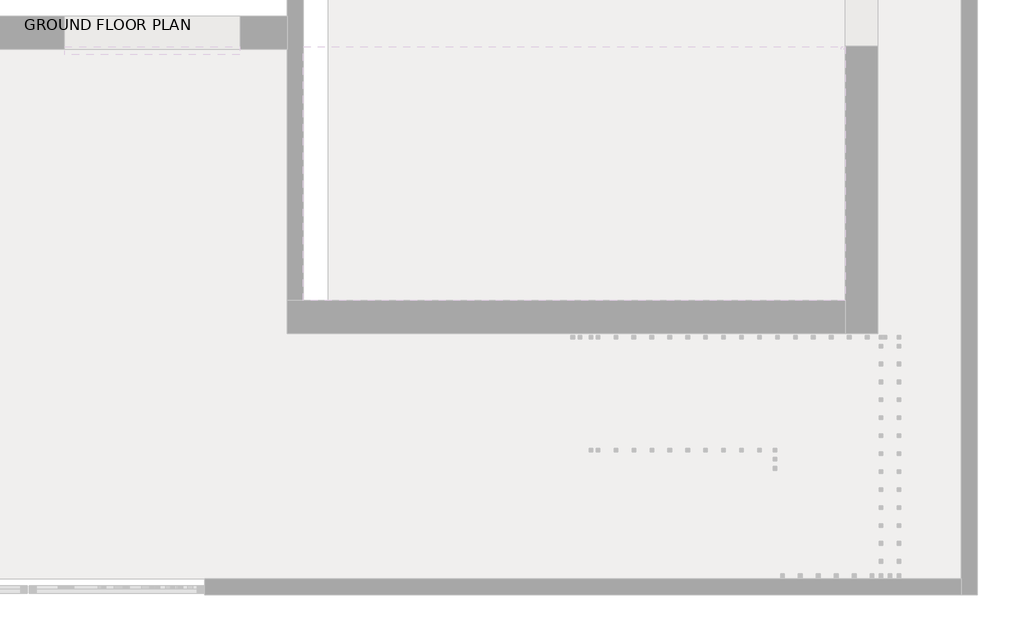
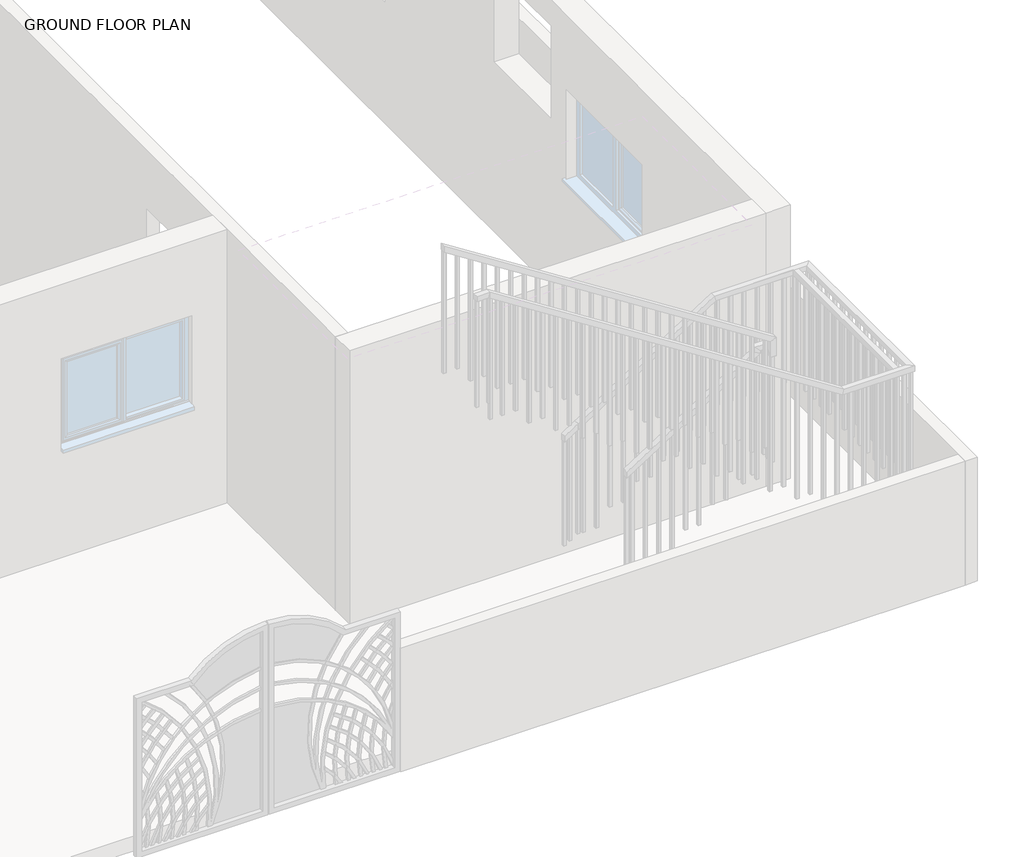
# One storey, part 13 of 23: 2 railings.
"""IFC4 building model written with IfcOpenShell, lengths in millimetres."""

from ifc_helpers import new_model, si_unit, frame, origin, place, context, project, spatial, polyline, outline, extrude, faceted_brep, element, save

model = new_model("IFC4")

# Units and contexts
model_context = context("Model", 3, world=origin())
ifc_project = project(units=[si_unit("LENGTHUNIT", "METRE", prefix="MILLI")], contexts=[model_context])

# Site, building, storey
site = spatial("IfcSite", under=ifc_project)
building = spatial("IfcBuilding", under=site)
storey = spatial("IfcBuildingStorey", under=building, Name="GROUND FLOOR PLAN", Elevation=487.68)

# Railings
placement = place(None, origin())
element("IfcRailing", 1, ObjectType="1100mm", at=placement, inside=storey, context=model_context, shape_type="SolidModel", body=[
    faceted_brep([(-8680.149573, -10220.0521308, 1912.8), (-8680.149573, -10220.0521308, 1853.4423995), (-8680.149573, -10270.0521308, 1853.4423995), (-8680.149573, -10270.0521308, 1912.8), (-7409.7306254, -10220.0521308, 2725.6), (-7395.1045513, -10220.0521308, 2675.6), (-7395.1045513, -10270.0521308, 2675.6), (-7409.7306254, -10270.0521308, 2725.6), (-6495.8132565, -10220.0521308, 2725.6), (-6495.8132565, -10220.0521308, 2675.6), (-6545.8132565, -10270.0521308, 2675.6), (-6545.8132565, -10270.0521308, 2725.6), (-6495.8132565, -11933.6860066, 2725.6), (-6495.8132565, -11933.6860066, 2675.6), (-6545.8132565, -11883.6860066, 2675.6), (-6545.8132565, -11883.6860066, 2725.6), (-7155.718398, -11933.6860066, 2725.6), (-7170.3479429, -11933.6860066, 2675.6), (-7170.3479429, -11883.6860066, 2675.6), (-7155.718398, -11883.6860066, 2725.6), (-10457.8773536, -11933.6860066, 4838.88), (-10457.8773536, -11883.6860066, 4838.88), (-10457.8773536, -11883.6860066, 4779.517542), (-10457.8773536, -11933.6860066, 4779.517542)], [[[0, 1, 2, 3]], [[1, 0, 4, 5]], [[2, 1, 5, 6]], [[3, 2, 6, 7]], [[0, 3, 7, 4]], [[5, 4, 8, 9]], [[6, 5, 9, 10]], [[7, 6, 10, 11]], [[4, 7, 11, 8]], [[9, 8, 12, 13]], [[10, 9, 13, 14]], [[11, 10, 14, 15]], [[8, 11, 15, 12]], [[13, 12, 16, 17]], [[14, 13, 17, 18]], [[15, 14, 18, 19]], [[12, 15, 19, 16]], [[20, 21, 22, 23]], [[17, 16, 20, 23]], [[18, 17, 23, 22]], [[19, 18, 22, 21]], [[16, 19, 21, 20]]]),
    extrude(outline(polyline([(4691.8007425, -10320.8132565), (4707.7999723, -10345.8132565), (3576.32, -10345.8132565), (3576.32, -10320.8132565), (4691.8007425, -10320.8132565)])), frame((0.0, -11921.1860066, 0.0), z_axis=(0.0, 1.0, 0.0), x_axis=(0.0, 0.0, 1.0)), (0.0, 0.0, 1.0), 25.0),
    extrude(outline(polyline([(4611.8045935, -10195.8132565), (4627.8038233, -10220.8132565), (3576.32, -10220.8132565), (3576.32, -10195.8132565), (4611.8045935, -10195.8132565)])), frame((0.0, -11921.1860066, 0.0), z_axis=(0.0, 1.0, 0.0), x_axis=(0.0, 0.0, 1.0)), (0.0, 0.0, 1.0), 25.0),
    extrude(outline(polyline([(4531.8084444, -10070.8132565), (4547.8076742, -10095.8132565), (3413.76, -10095.8132565), (3413.76, -10070.8132565), (4531.8084444, -10070.8132565)])), frame((0.0, -11921.1860066, 0.0), z_axis=(0.0, 1.0, 0.0), x_axis=(0.0, 0.0, 1.0)), (0.0, 0.0, 1.0), 25.0),
    extrude(outline(polyline([(4451.8122954, -9945.8132565), (4467.8115252, -9970.8132565), (3413.76, -9970.8132565), (3413.76, -9945.8132565), (4451.8122954, -9945.8132565)])), frame((0.0, -11921.1860066, 0.0), z_axis=(0.0, 1.0, 0.0), x_axis=(0.0, 0.0, 1.0)), (0.0, 0.0, 1.0), 25.0),
    extrude(outline(polyline([(4371.8161463, -9820.8132565), (4387.8153761, -9845.8132565), (3251.2, -9845.8132565), (3251.2, -9820.8132565), (4371.8161463, -9820.8132565)])), frame((0.0, -11921.1860066, 0.0), z_axis=(0.0, 1.0, 0.0), x_axis=(0.0, 0.0, 1.0)), (0.0, 0.0, 1.0), 25.0),
    extrude(outline(polyline([(4291.8423995, -9695.8132565), (4307.8371231, -9720.8132565), (3251.2, -9720.8132565), (3251.2, -9695.8132565), (4291.8423995, -9695.8132565)])), frame((0.0, -11921.1860066, 0.0), z_axis=(0.0, 1.0, 0.0), x_axis=(0.0, 0.0, 1.0)), (0.0, 0.0, 1.0), 25.0),
    extrude(outline(polyline([(4211.8238482, -9570.8132565), (4227.823078, -9595.8132565), (3088.64, -9595.8132565), (3088.64, -9570.8132565), (4211.8238482, -9570.8132565)])), frame((0.0, -11921.1860066, 0.0), z_axis=(0.0, 1.0, 0.0), x_axis=(0.0, 0.0, 1.0)), (0.0, 0.0, 1.0), 25.0),
    extrude(outline(polyline([(4131.8276992, -9445.8132565), (4147.826929, -9470.8132565), (3088.64, -9470.8132565), (3088.64, -9445.8132565), (4131.8276992, -9445.8132565)])), frame((0.0, -11921.1860066, 0.0), z_axis=(0.0, 1.0, 0.0), x_axis=(0.0, 0.0, 1.0)), (0.0, 0.0, 1.0), 25.0),
    extrude(outline(polyline([(4051.8315501, -9320.8132565), (4067.8307799, -9345.8132565), (2926.08, -9345.8132565), (2926.08, -9320.8132565), (4051.8315501, -9320.8132565)])), frame((0.0, -11921.1860066, 0.0), z_axis=(0.0, 1.0, 0.0), x_axis=(0.0, 0.0, 1.0)), (0.0, 0.0, 1.0), 25.0),
    extrude(outline(polyline([(3971.835401, -9195.8132565), (3987.8346309, -9220.8132565), (2926.08, -9220.8132565), (2926.08, -9195.8132565), (3971.835401, -9195.8132565)])), frame((0.0, -11921.1860066, 0.0), z_axis=(0.0, 1.0, 0.0), x_axis=(0.0, 0.0, 1.0)), (0.0, 0.0, 1.0), 25.0),
    extrude(outline(polyline([(3891.839252, -9070.8132565), (3907.8384818, -9095.8132565), (2763.52, -9095.8132565), (2763.52, -9070.8132565), (3891.839252, -9070.8132565)])), frame((0.0, -11921.1860066, 0.0), z_axis=(0.0, 1.0, 0.0), x_axis=(0.0, 0.0, 1.0)), (0.0, 0.0, 1.0), 25.0),
    extrude(outline(polyline([(3811.8431029, -8945.8132565), (3827.8423328, -8970.8132565), (2763.52, -8970.8132565), (2763.52, -8945.8132565), (3811.8431029, -8945.8132565)])), frame((0.0, -11921.1860066, 0.0), z_axis=(0.0, 1.0, 0.0), x_axis=(0.0, 0.0, 1.0)), (0.0, 0.0, 1.0), 25.0),
    extrude(outline(polyline([(3731.8469539, -8820.8132565), (3747.8461837, -8845.8132565), (2600.96, -8845.8132565), (2600.96, -8820.8132565), (3731.8469539, -8820.8132565)])), frame((0.0, -11921.1860066, 0.0), z_axis=(0.0, 1.0, 0.0), x_axis=(0.0, 0.0, 1.0)), (0.0, 0.0, 1.0), 25.0),
    extrude(outline(polyline([(3651.8508048, -8695.8132565), (3667.8500347, -8720.8132565), (2600.96, -8720.8132565), (2600.96, -8695.8132565), (3651.8508048, -8695.8132565)])), frame((0.0, -11921.1860066, 0.0), z_axis=(0.0, 1.0, 0.0), x_axis=(0.0, 0.0, 1.0)), (0.0, 0.0, 1.0), 25.0),
    extrude(outline(polyline([(3571.8546558, -8570.8132565), (3587.8538856, -8595.8132565), (2438.4, -8595.8132565), (2438.4, -8570.8132565), (3571.8546558, -8570.8132565)])), frame((0.0, -11921.1860066, 0.0), z_axis=(0.0, 1.0, 0.0), x_axis=(0.0, 0.0, 1.0)), (0.0, 0.0, 1.0), 25.0),
    extrude(outline(polyline([(3491.8585067, -8445.8132565), (3507.8577365, -8470.8132565), (2438.4, -8470.8132565), (2438.4, -8445.8132565), (3491.8585067, -8445.8132565)])), frame((0.0, -11921.1860066, 0.0), z_axis=(0.0, 1.0, 0.0), x_axis=(0.0, 0.0, 1.0)), (0.0, 0.0, 1.0), 25.0),
    extrude(outline(polyline([(3411.8623577, -8320.8132565), (3427.8615875, -8345.8132565), (2275.84, -8345.8132565), (2275.84, -8320.8132565), (3411.8623577, -8320.8132565)])), frame((0.0, -11921.1860066, 0.0), z_axis=(0.0, 1.0, 0.0), x_axis=(0.0, 0.0, 1.0)), (0.0, 0.0, 1.0), 25.0),
    extrude(outline(polyline([(3331.8662086, -8195.8132565), (3347.8654384, -8220.8132565), (2275.84, -8220.8132565), (2275.84, -8195.8132565), (3331.8662086, -8195.8132565)])), frame((0.0, -11921.1860066, 0.0), z_axis=(0.0, 1.0, 0.0), x_axis=(0.0, 0.0, 1.0)), (0.0, 0.0, 1.0), 25.0),
    extrude(outline(polyline([(3251.8700596, -8070.8132565), (3267.8692894, -8095.8132565), (2113.28, -8095.8132565), (2113.28, -8070.8132565), (3251.8700596, -8070.8132565)])), frame((0.0, -11921.1860066, 0.0), z_axis=(0.0, 1.0, 0.0), x_axis=(0.0, 0.0, 1.0)), (0.0, 0.0, 1.0), 25.0),
    extrude(outline(polyline([(3171.8739105, -7945.8132565), (3187.8731403, -7970.8132565), (2113.28, -7970.8132565), (2113.28, -7945.8132565), (3171.8739105, -7945.8132565)])), frame((0.0, -11921.1860066, 0.0), z_axis=(0.0, 1.0, 0.0), x_axis=(0.0, 0.0, 1.0)), (0.0, 0.0, 1.0), 25.0),
    extrude(outline(polyline([(3091.8777615, -7820.8132565), (3107.8769913, -7845.8132565), (1950.72, -7845.8132565), (1950.72, -7820.8132565), (3091.8777615, -7820.8132565)])), frame((0.0, -11921.1860066, 0.0), z_axis=(0.0, 1.0, 0.0), x_axis=(0.0, 0.0, 1.0)), (0.0, 0.0, 1.0), 25.0),
    extrude(outline(polyline([(3011.8816124, -7695.8132565), (3027.8808422, -7720.8132565), (1950.72, -7720.8132565), (1950.72, -7695.8132565), (3011.8816124, -7695.8132565)])), frame((0.0, -11921.1860066, 0.0), z_axis=(0.0, 1.0, 0.0), x_axis=(0.0, 0.0, 1.0)), (0.0, 0.0, 1.0), 25.0),
    extrude(outline(polyline([(2931.8854634, -7570.8132565), (2947.8846932, -7595.8132565), (1788.16, -7595.8132565), (1788.16, -7570.8132565), (2931.8854634, -7570.8132565)])), frame((0.0, -11921.1860066, 0.0), z_axis=(0.0, 1.0, 0.0), x_axis=(0.0, 0.0, 1.0)), (0.0, 0.0, 1.0), 25.0),
    extrude(outline(polyline([(2851.8893143, -7445.8132565), (2867.8885441, -7470.8132565), (1788.16, -7470.8132565), (1788.16, -7445.8132565), (2851.8893143, -7445.8132565)])), frame((0.0, -11921.1860066, 0.0), z_axis=(0.0, 1.0, 0.0), x_axis=(0.0, 0.0, 1.0)), (0.0, 0.0, 1.0), 25.0),
    extrude(outline(polyline([(2771.8931653, -7320.8132565), (2787.8923951, -7345.8132565), (1625.6, -7345.8132565), (1625.6, -7320.8132565), (2771.8931653, -7320.8132565)])), frame((0.0, -11921.1860066, 0.0), z_axis=(0.0, 1.0, 0.0), x_axis=(0.0, 0.0, 1.0)), (0.0, 0.0, 1.0), 25.0),
    extrude(outline(polyline([(2691.8970162, -7195.8132565), (2707.896246, -7220.8132565), (1625.6, -7220.8132565), (1625.6, -7195.8132565), (2691.8970162, -7195.8132565)])), frame((0.0, -11921.1860066, 0.0), z_axis=(0.0, 1.0, 0.0), x_axis=(0.0, 0.0, 1.0)), (0.0, 0.0, 1.0), 25.0),
    extrude(outline(polyline([(-7070.8132565, -11921.1860066), (-7095.8132565, -11921.1860066), (-7095.8132565, -11896.1860066), (-7070.8132565, -11896.1860066), (-7070.8132565, -11921.1860066)])), frame((0.0, 0.0, 1625.6), z_axis=(0.0, 0.0, 1.0), x_axis=(1.0, 0.0, 0.0)), (0.0, 0.0, 1.0), 1050.0),
    extrude(outline(polyline([(-6945.8132565, -11921.1860066), (-6970.8132565, -11921.1860066), (-6970.8132565, -11896.1860066), (-6945.8132565, -11896.1860066), (-6945.8132565, -11921.1860066)])), frame((0.0, 0.0, 1625.6), z_axis=(0.0, 0.0, 1.0), x_axis=(1.0, 0.0, 0.0)), (0.0, 0.0, 1.0), 1050.0),
    extrude(outline(polyline([(-6820.8132565, -11921.1860066), (-6845.8132565, -11921.1860066), (-6845.8132565, -11896.1860066), (-6820.8132565, -11896.1860066), (-6820.8132565, -11921.1860066)])), frame((0.0, 0.0, 1625.6), z_axis=(0.0, 0.0, 1.0), x_axis=(1.0, 0.0, 0.0)), (0.0, 0.0, 1.0), 1050.0),
    extrude(outline(polyline([(-6695.8132565, -11921.1860066), (-6720.8132565, -11921.1860066), (-6720.8132565, -11896.1860066), (-6695.8132565, -11896.1860066), (-6695.8132565, -11921.1860066)])), frame((0.0, 0.0, 1625.6), z_axis=(0.0, 0.0, 1.0), x_axis=(1.0, 0.0, 0.0)), (0.0, 0.0, 1.0), 1050.0),
    extrude(outline(polyline([(-6570.8132565, -11921.1860066), (-6595.8132565, -11921.1860066), (-6595.8132565, -11896.1860066), (-6570.8132565, -11896.1860066), (-6570.8132565, -11921.1860066)])), frame((0.0, 0.0, 1625.6), z_axis=(0.0, 0.0, 1.0), x_axis=(1.0, 0.0, 0.0)), (0.0, 0.0, 1.0), 1050.0),
    extrude(outline(polyline([(-6508.3132565, -11795.0521308), (-6508.3132565, -11820.0521308), (-6533.3132565, -11820.0521308), (-6533.3132565, -11795.0521308), (-6508.3132565, -11795.0521308)])), frame((0.0, 0.0, 1625.6), z_axis=(0.0, 0.0, 1.0), x_axis=(1.0, 0.0, 0.0)), (0.0, 0.0, 1.0), 1050.0),
    extrude(outline(polyline([(-6508.3132565, -11670.0521308), (-6508.3132565, -11695.0521308), (-6533.3132565, -11695.0521308), (-6533.3132565, -11670.0521308), (-6508.3132565, -11670.0521308)])), frame((0.0, 0.0, 1625.6), z_axis=(0.0, 0.0, 1.0), x_axis=(1.0, 0.0, 0.0)), (0.0, 0.0, 1.0), 1050.0),
    extrude(outline(polyline([(-6508.3132565, -11545.0521308), (-6508.3132565, -11570.0521308), (-6533.3132565, -11570.0521308), (-6533.3132565, -11545.0521308), (-6508.3132565, -11545.0521308)])), frame((0.0, 0.0, 1625.6), z_axis=(0.0, 0.0, 1.0), x_axis=(1.0, 0.0, 0.0)), (0.0, 0.0, 1.0), 1050.0),
    extrude(outline(polyline([(-6508.3132565, -11420.0521308), (-6508.3132565, -11445.0521308), (-6533.3132565, -11445.0521308), (-6533.3132565, -11420.0521308), (-6508.3132565, -11420.0521308)])), frame((0.0, 0.0, 1625.6), z_axis=(0.0, 0.0, 1.0), x_axis=(1.0, 0.0, 0.0)), (0.0, 0.0, 1.0), 1050.0),
    extrude(outline(polyline([(-6508.3132565, -11295.0521308), (-6508.3132565, -11320.0521308), (-6533.3132565, -11320.0521308), (-6533.3132565, -11295.0521308), (-6508.3132565, -11295.0521308)])), frame((0.0, 0.0, 1625.6), z_axis=(0.0, 0.0, 1.0), x_axis=(1.0, 0.0, 0.0)), (0.0, 0.0, 1.0), 1050.0),
    extrude(outline(polyline([(-6508.3132565, -11170.0521308), (-6508.3132565, -11195.0521308), (-6533.3132565, -11195.0521308), (-6533.3132565, -11170.0521308), (-6508.3132565, -11170.0521308)])), frame((0.0, 0.0, 1625.6), z_axis=(0.0, 0.0, 1.0), x_axis=(1.0, 0.0, 0.0)), (0.0, 0.0, 1.0), 1050.0),
    extrude(outline(polyline([(-6508.3132565, -11045.0521308), (-6508.3132565, -11070.0521308), (-6533.3132565, -11070.0521308), (-6533.3132565, -11045.0521308), (-6508.3132565, -11045.0521308)])), frame((0.0, 0.0, 1625.6), z_axis=(0.0, 0.0, 1.0), x_axis=(1.0, 0.0, 0.0)), (0.0, 0.0, 1.0), 1050.0),
    extrude(outline(polyline([(-6508.3132565, -10920.0521308), (-6508.3132565, -10945.0521308), (-6533.3132565, -10945.0521308), (-6533.3132565, -10920.0521308), (-6508.3132565, -10920.0521308)])), frame((0.0, 0.0, 1625.6), z_axis=(0.0, 0.0, 1.0), x_axis=(1.0, 0.0, 0.0)), (0.0, 0.0, 1.0), 1050.0),
    extrude(outline(polyline([(-6508.3132565, -10795.0521308), (-6508.3132565, -10820.0521308), (-6533.3132565, -10820.0521308), (-6533.3132565, -10795.0521308), (-6508.3132565, -10795.0521308)])), frame((0.0, 0.0, 1625.6), z_axis=(0.0, 0.0, 1.0), x_axis=(1.0, 0.0, 0.0)), (0.0, 0.0, 1.0), 1050.0),
    extrude(outline(polyline([(-6508.3132565, -10670.0521308), (-6508.3132565, -10695.0521308), (-6533.3132565, -10695.0521308), (-6533.3132565, -10670.0521308), (-6508.3132565, -10670.0521308)])), frame((0.0, 0.0, 1625.6), z_axis=(0.0, 0.0, 1.0), x_axis=(1.0, 0.0, 0.0)), (0.0, 0.0, 1.0), 1050.0),
    extrude(outline(polyline([(-6508.3132565, -10545.0521308), (-6508.3132565, -10570.0521308), (-6533.3132565, -10570.0521308), (-6533.3132565, -10545.0521308), (-6508.3132565, -10545.0521308)])), frame((0.0, 0.0, 1625.6), z_axis=(0.0, 0.0, 1.0), x_axis=(1.0, 0.0, 0.0)), (0.0, 0.0, 1.0), 1050.0),
    extrude(outline(polyline([(-6508.3132565, -10420.0521308), (-6508.3132565, -10445.0521308), (-6533.3132565, -10445.0521308), (-6533.3132565, -10420.0521308), (-6508.3132565, -10420.0521308)])), frame((0.0, 0.0, 1625.6), z_axis=(0.0, 0.0, 1.0), x_axis=(1.0, 0.0, 0.0)), (0.0, 0.0, 1.0), 1050.0),
    extrude(outline(polyline([(-6508.3132565, -10295.0521308), (-6508.3132565, -10320.0521308), (-6533.3132565, -10320.0521308), (-6533.3132565, -10295.0521308), (-6508.3132565, -10295.0521308)])), frame((0.0, 0.0, 1625.6), z_axis=(0.0, 0.0, 1.0), x_axis=(1.0, 0.0, 0.0)), (0.0, 0.0, 1.0), 1050.0),
    extrude(outline(polyline([(-6630.149573, -10232.5521308), (-6605.149573, -10232.5521308), (-6605.149573, -10257.5521308), (-6630.149573, -10257.5521308), (-6630.149573, -10232.5521308)])), frame((0.0, 0.0, 1625.6), z_axis=(0.0, 0.0, 1.0), x_axis=(1.0, 0.0, 0.0)), (0.0, 0.0, 1.0), 1050.0),
    extrude(outline(polyline([(-6755.149573, -10232.5521308), (-6730.149573, -10232.5521308), (-6730.149573, -10257.5521308), (-6755.149573, -10257.5521308), (-6755.149573, -10232.5521308)])), frame((0.0, 0.0, 1625.6), z_axis=(0.0, 0.0, 1.0), x_axis=(1.0, 0.0, 0.0)), (0.0, 0.0, 1.0), 1050.0),
    extrude(outline(polyline([(-6880.149573, -10232.5521308), (-6855.149573, -10232.5521308), (-6855.149573, -10257.5521308), (-6880.149573, -10257.5521308), (-6880.149573, -10232.5521308)])), frame((0.0, 0.0, 1625.6), z_axis=(0.0, 0.0, 1.0), x_axis=(1.0, 0.0, 0.0)), (0.0, 0.0, 1.0), 1050.0),
    extrude(outline(polyline([(-7005.149573, -10232.5521308), (-6980.149573, -10232.5521308), (-6980.149573, -10257.5521308), (-7005.149573, -10257.5521308), (-7005.149573, -10232.5521308)])), frame((0.0, 0.0, 1625.6), z_axis=(0.0, 0.0, 1.0), x_axis=(1.0, 0.0, 0.0)), (0.0, 0.0, 1.0), 1050.0),
    extrude(outline(polyline([(-7130.149573, -10232.5521308), (-7105.149573, -10232.5521308), (-7105.149573, -10257.5521308), (-7130.149573, -10257.5521308), (-7130.149573, -10232.5521308)])), frame((0.0, 0.0, 1625.6), z_axis=(0.0, 0.0, 1.0), x_axis=(1.0, 0.0, 0.0)), (0.0, 0.0, 1.0), 1050.0),
    extrude(outline(polyline([(-7255.149573, -10232.5521308), (-7230.149573, -10232.5521308), (-7230.149573, -10257.5521308), (-7255.149573, -10257.5521308), (-7255.149573, -10232.5521308)])), frame((0.0, 0.0, 1625.6), z_axis=(0.0, 0.0, 1.0), x_axis=(1.0, 0.0, 0.0)), (0.0, 0.0, 1.0), 1050.0),
    extrude(outline(polyline([(-7380.149573, -10232.5521308), (-7355.149573, -10232.5521308), (-7355.149573, -10257.5521308), (-7380.149573, -10257.5521308), (-7380.149573, -10232.5521308)])), frame((0.0, 0.0, 1625.6), z_axis=(0.0, 0.0, 1.0), x_axis=(1.0, 0.0, 0.0)), (0.0, 0.0, 1.0), 1050.0),
    extrude(outline(polyline([(1463.04, -7505.149573), (1463.04, -7480.149573), (2621.1891352, -7480.149573), (2605.1944115, -7505.149573), (1463.04, -7505.149573)])), frame((0.0, -10257.5521308, 0.0), z_axis=(0.0, 1.0, 0.0), x_axis=(0.0, 0.0, 1.0)), (0.0, 0.0, 1.0), 25.0),
    extrude(outline(polyline([(1463.04, -7630.149573), (1463.04, -7605.149573), (2541.2155169, -7605.149573), (2525.2207932, -7630.149573), (1463.04, -7630.149573)])), frame((0.0, -10257.5521308, 0.0), z_axis=(0.0, 1.0, 0.0), x_axis=(0.0, 0.0, 1.0)), (0.0, 0.0, 1.0), 25.0),
    extrude(outline(polyline([(1300.48, -7755.149573), (1300.48, -7730.149573), (2461.2418986, -7730.149573), (2445.2471749, -7755.149573), (1300.48, -7755.149573)])), frame((0.0, -10257.5521308, 0.0), z_axis=(0.0, 1.0, 0.0), x_axis=(0.0, 0.0, 1.0)), (0.0, 0.0, 1.0), 25.0),
    extrude(outline(polyline([(1300.48, -7880.149573), (1300.48, -7855.149573), (2381.2682803, -7855.149573), (2365.2735566, -7880.149573), (1300.48, -7880.149573)])), frame((0.0, -10257.5521308, 0.0), z_axis=(0.0, 1.0, 0.0), x_axis=(0.0, 0.0, 1.0)), (0.0, 0.0, 1.0), 25.0),
    extrude(outline(polyline([(1137.92, -8005.149573), (1137.92, -7980.149573), (2301.294662, -7980.149573), (2285.2999383, -8005.149573), (1137.92, -8005.149573)])), frame((0.0, -10257.5521308, 0.0), z_axis=(0.0, 1.0, 0.0), x_axis=(0.0, 0.0, 1.0)), (0.0, 0.0, 1.0), 25.0),
    extrude(outline(polyline([(1137.92, -8130.149573), (1137.92, -8105.149573), (2221.3210437, -8105.149573), (2205.32632, -8130.149573), (1137.92, -8130.149573)])), frame((0.0, -10257.5521308, 0.0), z_axis=(0.0, 1.0, 0.0), x_axis=(0.0, 0.0, 1.0)), (0.0, 0.0, 1.0), 25.0),
    extrude(outline(polyline([(975.36, -8255.149573), (975.36, -8230.149573), (2141.3474254, -8230.149573), (2125.3527017, -8255.149573), (975.36, -8255.149573)])), frame((0.0, -10257.5521308, 0.0), z_axis=(0.0, 1.0, 0.0), x_axis=(0.0, 0.0, 1.0)), (0.0, 0.0, 1.0), 25.0),
    extrude(outline(polyline([(975.36, -8380.149573), (975.36, -8355.149573), (2061.3738071, -8355.149573), (2045.3790834, -8380.149573), (975.36, -8380.149573)])), frame((0.0, -10257.5521308, 0.0), z_axis=(0.0, 1.0, 0.0), x_axis=(0.0, 0.0, 1.0)), (0.0, 0.0, 1.0), 25.0),
    extrude(outline(polyline([(812.8, -8505.149573), (812.8, -8480.149573), (1981.4001888, -8480.149573), (1965.4054651, -8505.149573), (812.8, -8505.149573)])), frame((0.0, -10257.5521308, 0.0), z_axis=(0.0, 1.0, 0.0), x_axis=(0.0, 0.0, 1.0)), (0.0, 0.0, 1.0), 25.0),
    extrude(outline(polyline([(812.8, -8630.149573), (812.8, -8605.149573), (1901.4265705, -8605.149573), (1885.4318468, -8630.149573), (812.8, -8630.149573)])), frame((0.0, -10257.5521308, 0.0), z_axis=(0.0, 1.0, 0.0), x_axis=(0.0, 0.0, 1.0)), (0.0, 0.0, 1.0), 25.0),
    extrude(outline(polyline([(-6508.3132565, -11896.1860066), (-6508.3132565, -11921.1860066), (-6533.3132565, -11921.1860066), (-6533.3132565, -11896.1860066), (-6508.3132565, -11896.1860066)])), frame((0.0, 0.0, 1625.6), z_axis=(0.0, 0.0, 1.0), x_axis=(1.0, 0.0, 0.0)), (0.0, 0.0, 1.0), 1050.0),
    extrude(outline(polyline([(-6533.3132565, -10232.5521308), (-6508.3132565, -10232.5521308), (-6508.3132565, -10257.5521308), (-6533.3132565, -10257.5521308), (-6533.3132565, -10232.5521308)])), frame((0.0, 0.0, 1625.6), z_axis=(0.0, 0.0, 1.0), x_axis=(1.0, 0.0, 0.0)), (0.0, 0.0, 1.0), 1050.0),
    extrude(outline(polyline([(4763.5183122, -10432.8773536), (4779.517542, -10457.8773536), (3576.32, -10457.8773536), (3576.32, -10432.8773536), (4763.5183122, -10432.8773536)])), frame((0.0, -11921.1860066, 0.0), z_axis=(0.0, 1.0, 0.0), x_axis=(0.0, 0.0, 1.0)), (0.0, 0.0, 1.0), 25.0),
    extrude(outline(polyline([(812.8, -8680.149573), (812.8, -8655.149573), (1869.4371231, -8655.149573), (1853.4423995, -8680.149573), (812.8, -8680.149573)])), frame((0.0, -10257.5521308, 0.0), z_axis=(0.0, 1.0, 0.0), x_axis=(0.0, 0.0, 1.0)), (0.0, 0.0, 1.0), 25.0),
])
element("IfcRailing", 2, ObjectType="1100mm", at=placement, inside=storey, context=model_context, shape_type="SolidModel", body=[
    faceted_brep([(-8680.149573, -10220.0521308, 1912.8), (-8680.149573, -10220.0521308, 1853.4423995), (-8680.149573, -10270.0521308, 1853.4423995), (-8680.149573, -10270.0521308, 1912.8), (-7409.7306254, -10220.0521308, 2725.6), (-7395.1045513, -10220.0521308, 2675.6), (-7395.1045513, -10270.0521308, 2675.6), (-7409.7306254, -10270.0521308, 2725.6), (-6495.8132565, -10220.0521308, 2725.6), (-6495.8132565, -10220.0521308, 2675.6), (-6545.8132565, -10270.0521308, 2675.6), (-6545.8132565, -10270.0521308, 2725.6), (-6495.8132565, -11933.6860066, 2725.6), (-6495.8132565, -11933.6860066, 2675.6), (-6545.8132565, -11883.6860066, 2675.6), (-6545.8132565, -11883.6860066, 2725.6), (-7155.718398, -11933.6860066, 2725.6), (-7170.3479429, -11933.6860066, 2675.6), (-7170.3479429, -11883.6860066, 2675.6), (-7155.718398, -11883.6860066, 2725.6), (-10457.8773536, -11933.6860066, 4838.88), (-10457.8773536, -11883.6860066, 4838.88), (-10457.8773536, -11883.6860066, 4779.517542), (-10457.8773536, -11933.6860066, 4779.517542)], [[[0, 1, 2, 3]], [[1, 0, 4, 5]], [[2, 1, 5, 6]], [[3, 2, 6, 7]], [[0, 3, 7, 4]], [[5, 4, 8, 9]], [[6, 5, 9, 10]], [[7, 6, 10, 11]], [[4, 7, 11, 8]], [[9, 8, 12, 13]], [[10, 9, 13, 14]], [[11, 10, 14, 15]], [[8, 11, 15, 12]], [[13, 12, 16, 17]], [[14, 13, 17, 18]], [[15, 14, 18, 19]], [[12, 15, 19, 16]], [[20, 21, 22, 23]], [[17, 16, 20, 23]], [[18, 17, 23, 22]], [[19, 18, 22, 21]], [[16, 19, 21, 20]]]),
    extrude(outline(polyline([(4691.8007425, -10320.8132565), (4707.7999723, -10345.8132565), (3576.32, -10345.8132565), (3576.32, -10320.8132565), (4691.8007425, -10320.8132565)])), frame((0.0, -11921.1860066, 0.0), z_axis=(0.0, 1.0, 0.0), x_axis=(0.0, 0.0, 1.0)), (0.0, 0.0, 1.0), 25.0),
    extrude(outline(polyline([(4611.8045935, -10195.8132565), (4627.8038233, -10220.8132565), (3576.32, -10220.8132565), (3576.32, -10195.8132565), (4611.8045935, -10195.8132565)])), frame((0.0, -11921.1860066, 0.0), z_axis=(0.0, 1.0, 0.0), x_axis=(0.0, 0.0, 1.0)), (0.0, 0.0, 1.0), 25.0),
    extrude(outline(polyline([(4531.8084444, -10070.8132565), (4547.8076742, -10095.8132565), (3413.76, -10095.8132565), (3413.76, -10070.8132565), (4531.8084444, -10070.8132565)])), frame((0.0, -11921.1860066, 0.0), z_axis=(0.0, 1.0, 0.0), x_axis=(0.0, 0.0, 1.0)), (0.0, 0.0, 1.0), 25.0),
    extrude(outline(polyline([(4451.8122954, -9945.8132565), (4467.8115252, -9970.8132565), (3413.76, -9970.8132565), (3413.76, -9945.8132565), (4451.8122954, -9945.8132565)])), frame((0.0, -11921.1860066, 0.0), z_axis=(0.0, 1.0, 0.0), x_axis=(0.0, 0.0, 1.0)), (0.0, 0.0, 1.0), 25.0),
    extrude(outline(polyline([(4371.8161463, -9820.8132565), (4387.8153761, -9845.8132565), (3251.2, -9845.8132565), (3251.2, -9820.8132565), (4371.8161463, -9820.8132565)])), frame((0.0, -11921.1860066, 0.0), z_axis=(0.0, 1.0, 0.0), x_axis=(0.0, 0.0, 1.0)), (0.0, 0.0, 1.0), 25.0),
    extrude(outline(polyline([(4291.8423995, -9695.8132565), (4307.8371231, -9720.8132565), (3251.2, -9720.8132565), (3251.2, -9695.8132565), (4291.8423995, -9695.8132565)])), frame((0.0, -11921.1860066, 0.0), z_axis=(0.0, 1.0, 0.0), x_axis=(0.0, 0.0, 1.0)), (0.0, 0.0, 1.0), 25.0),
    extrude(outline(polyline([(4211.8238482, -9570.8132565), (4227.823078, -9595.8132565), (3088.64, -9595.8132565), (3088.64, -9570.8132565), (4211.8238482, -9570.8132565)])), frame((0.0, -11921.1860066, 0.0), z_axis=(0.0, 1.0, 0.0), x_axis=(0.0, 0.0, 1.0)), (0.0, 0.0, 1.0), 25.0),
    extrude(outline(polyline([(4131.8276992, -9445.8132565), (4147.826929, -9470.8132565), (3088.64, -9470.8132565), (3088.64, -9445.8132565), (4131.8276992, -9445.8132565)])), frame((0.0, -11921.1860066, 0.0), z_axis=(0.0, 1.0, 0.0), x_axis=(0.0, 0.0, 1.0)), (0.0, 0.0, 1.0), 25.0),
    extrude(outline(polyline([(4051.8315501, -9320.8132565), (4067.8307799, -9345.8132565), (2926.08, -9345.8132565), (2926.08, -9320.8132565), (4051.8315501, -9320.8132565)])), frame((0.0, -11921.1860066, 0.0), z_axis=(0.0, 1.0, 0.0), x_axis=(0.0, 0.0, 1.0)), (0.0, 0.0, 1.0), 25.0),
    extrude(outline(polyline([(3971.835401, -9195.8132565), (3987.8346309, -9220.8132565), (2926.08, -9220.8132565), (2926.08, -9195.8132565), (3971.835401, -9195.8132565)])), frame((0.0, -11921.1860066, 0.0), z_axis=(0.0, 1.0, 0.0), x_axis=(0.0, 0.0, 1.0)), (0.0, 0.0, 1.0), 25.0),
    extrude(outline(polyline([(3891.839252, -9070.8132565), (3907.8384818, -9095.8132565), (2763.52, -9095.8132565), (2763.52, -9070.8132565), (3891.839252, -9070.8132565)])), frame((0.0, -11921.1860066, 0.0), z_axis=(0.0, 1.0, 0.0), x_axis=(0.0, 0.0, 1.0)), (0.0, 0.0, 1.0), 25.0),
    extrude(outline(polyline([(3811.8431029, -8945.8132565), (3827.8423328, -8970.8132565), (2763.52, -8970.8132565), (2763.52, -8945.8132565), (3811.8431029, -8945.8132565)])), frame((0.0, -11921.1860066, 0.0), z_axis=(0.0, 1.0, 0.0), x_axis=(0.0, 0.0, 1.0)), (0.0, 0.0, 1.0), 25.0),
    extrude(outline(polyline([(3731.8469539, -8820.8132565), (3747.8461837, -8845.8132565), (2600.96, -8845.8132565), (2600.96, -8820.8132565), (3731.8469539, -8820.8132565)])), frame((0.0, -11921.1860066, 0.0), z_axis=(0.0, 1.0, 0.0), x_axis=(0.0, 0.0, 1.0)), (0.0, 0.0, 1.0), 25.0),
    extrude(outline(polyline([(3651.8508048, -8695.8132565), (3667.8500347, -8720.8132565), (2600.96, -8720.8132565), (2600.96, -8695.8132565), (3651.8508048, -8695.8132565)])), frame((0.0, -11921.1860066, 0.0), z_axis=(0.0, 1.0, 0.0), x_axis=(0.0, 0.0, 1.0)), (0.0, 0.0, 1.0), 25.0),
    extrude(outline(polyline([(3571.8546558, -8570.8132565), (3587.8538856, -8595.8132565), (2438.4, -8595.8132565), (2438.4, -8570.8132565), (3571.8546558, -8570.8132565)])), frame((0.0, -11921.1860066, 0.0), z_axis=(0.0, 1.0, 0.0), x_axis=(0.0, 0.0, 1.0)), (0.0, 0.0, 1.0), 25.0),
    extrude(outline(polyline([(3491.8585067, -8445.8132565), (3507.8577365, -8470.8132565), (2438.4, -8470.8132565), (2438.4, -8445.8132565), (3491.8585067, -8445.8132565)])), frame((0.0, -11921.1860066, 0.0), z_axis=(0.0, 1.0, 0.0), x_axis=(0.0, 0.0, 1.0)), (0.0, 0.0, 1.0), 25.0),
    extrude(outline(polyline([(3411.8623577, -8320.8132565), (3427.8615875, -8345.8132565), (2275.84, -8345.8132565), (2275.84, -8320.8132565), (3411.8623577, -8320.8132565)])), frame((0.0, -11921.1860066, 0.0), z_axis=(0.0, 1.0, 0.0), x_axis=(0.0, 0.0, 1.0)), (0.0, 0.0, 1.0), 25.0),
    extrude(outline(polyline([(3331.8662086, -8195.8132565), (3347.8654384, -8220.8132565), (2275.84, -8220.8132565), (2275.84, -8195.8132565), (3331.8662086, -8195.8132565)])), frame((0.0, -11921.1860066, 0.0), z_axis=(0.0, 1.0, 0.0), x_axis=(0.0, 0.0, 1.0)), (0.0, 0.0, 1.0), 25.0),
    extrude(outline(polyline([(3251.8700596, -8070.8132565), (3267.8692894, -8095.8132565), (2113.28, -8095.8132565), (2113.28, -8070.8132565), (3251.8700596, -8070.8132565)])), frame((0.0, -11921.1860066, 0.0), z_axis=(0.0, 1.0, 0.0), x_axis=(0.0, 0.0, 1.0)), (0.0, 0.0, 1.0), 25.0),
    extrude(outline(polyline([(3171.8739105, -7945.8132565), (3187.8731403, -7970.8132565), (2113.28, -7970.8132565), (2113.28, -7945.8132565), (3171.8739105, -7945.8132565)])), frame((0.0, -11921.1860066, 0.0), z_axis=(0.0, 1.0, 0.0), x_axis=(0.0, 0.0, 1.0)), (0.0, 0.0, 1.0), 25.0),
    extrude(outline(polyline([(3091.8777615, -7820.8132565), (3107.8769913, -7845.8132565), (1950.72, -7845.8132565), (1950.72, -7820.8132565), (3091.8777615, -7820.8132565)])), frame((0.0, -11921.1860066, 0.0), z_axis=(0.0, 1.0, 0.0), x_axis=(0.0, 0.0, 1.0)), (0.0, 0.0, 1.0), 25.0),
    extrude(outline(polyline([(3011.8816124, -7695.8132565), (3027.8808422, -7720.8132565), (1950.72, -7720.8132565), (1950.72, -7695.8132565), (3011.8816124, -7695.8132565)])), frame((0.0, -11921.1860066, 0.0), z_axis=(0.0, 1.0, 0.0), x_axis=(0.0, 0.0, 1.0)), (0.0, 0.0, 1.0), 25.0),
    extrude(outline(polyline([(2931.8854634, -7570.8132565), (2947.8846932, -7595.8132565), (1788.16, -7595.8132565), (1788.16, -7570.8132565), (2931.8854634, -7570.8132565)])), frame((0.0, -11921.1860066, 0.0), z_axis=(0.0, 1.0, 0.0), x_axis=(0.0, 0.0, 1.0)), (0.0, 0.0, 1.0), 25.0),
    extrude(outline(polyline([(2851.8893143, -7445.8132565), (2867.8885441, -7470.8132565), (1788.16, -7470.8132565), (1788.16, -7445.8132565), (2851.8893143, -7445.8132565)])), frame((0.0, -11921.1860066, 0.0), z_axis=(0.0, 1.0, 0.0), x_axis=(0.0, 0.0, 1.0)), (0.0, 0.0, 1.0), 25.0),
    extrude(outline(polyline([(2771.8931653, -7320.8132565), (2787.8923951, -7345.8132565), (1625.6, -7345.8132565), (1625.6, -7320.8132565), (2771.8931653, -7320.8132565)])), frame((0.0, -11921.1860066, 0.0), z_axis=(0.0, 1.0, 0.0), x_axis=(0.0, 0.0, 1.0)), (0.0, 0.0, 1.0), 25.0),
    extrude(outline(polyline([(2691.8970162, -7195.8132565), (2707.896246, -7220.8132565), (1625.6, -7220.8132565), (1625.6, -7195.8132565), (2691.8970162, -7195.8132565)])), frame((0.0, -11921.1860066, 0.0), z_axis=(0.0, 1.0, 0.0), x_axis=(0.0, 0.0, 1.0)), (0.0, 0.0, 1.0), 25.0),
    extrude(outline(polyline([(-7070.8132565, -11921.1860066), (-7095.8132565, -11921.1860066), (-7095.8132565, -11896.1860066), (-7070.8132565, -11896.1860066), (-7070.8132565, -11921.1860066)])), frame((0.0, 0.0, 1625.6), z_axis=(0.0, 0.0, 1.0), x_axis=(1.0, 0.0, 0.0)), (0.0, 0.0, 1.0), 1050.0),
    extrude(outline(polyline([(-6945.8132565, -11921.1860066), (-6970.8132565, -11921.1860066), (-6970.8132565, -11896.1860066), (-6945.8132565, -11896.1860066), (-6945.8132565, -11921.1860066)])), frame((0.0, 0.0, 1625.6), z_axis=(0.0, 0.0, 1.0), x_axis=(1.0, 0.0, 0.0)), (0.0, 0.0, 1.0), 1050.0),
    extrude(outline(polyline([(-6820.8132565, -11921.1860066), (-6845.8132565, -11921.1860066), (-6845.8132565, -11896.1860066), (-6820.8132565, -11896.1860066), (-6820.8132565, -11921.1860066)])), frame((0.0, 0.0, 1625.6), z_axis=(0.0, 0.0, 1.0), x_axis=(1.0, 0.0, 0.0)), (0.0, 0.0, 1.0), 1050.0),
    extrude(outline(polyline([(-6695.8132565, -11921.1860066), (-6720.8132565, -11921.1860066), (-6720.8132565, -11896.1860066), (-6695.8132565, -11896.1860066), (-6695.8132565, -11921.1860066)])), frame((0.0, 0.0, 1625.6), z_axis=(0.0, 0.0, 1.0), x_axis=(1.0, 0.0, 0.0)), (0.0, 0.0, 1.0), 1050.0),
    extrude(outline(polyline([(-6570.8132565, -11921.1860066), (-6595.8132565, -11921.1860066), (-6595.8132565, -11896.1860066), (-6570.8132565, -11896.1860066), (-6570.8132565, -11921.1860066)])), frame((0.0, 0.0, 1625.6), z_axis=(0.0, 0.0, 1.0), x_axis=(1.0, 0.0, 0.0)), (0.0, 0.0, 1.0), 1050.0),
    extrude(outline(polyline([(-6508.3132565, -11795.0521308), (-6508.3132565, -11820.0521308), (-6533.3132565, -11820.0521308), (-6533.3132565, -11795.0521308), (-6508.3132565, -11795.0521308)])), frame((0.0, 0.0, 1625.6), z_axis=(0.0, 0.0, 1.0), x_axis=(1.0, 0.0, 0.0)), (0.0, 0.0, 1.0), 1050.0),
    extrude(outline(polyline([(-6508.3132565, -11670.0521308), (-6508.3132565, -11695.0521308), (-6533.3132565, -11695.0521308), (-6533.3132565, -11670.0521308), (-6508.3132565, -11670.0521308)])), frame((0.0, 0.0, 1625.6), z_axis=(0.0, 0.0, 1.0), x_axis=(1.0, 0.0, 0.0)), (0.0, 0.0, 1.0), 1050.0),
    extrude(outline(polyline([(-6508.3132565, -11545.0521308), (-6508.3132565, -11570.0521308), (-6533.3132565, -11570.0521308), (-6533.3132565, -11545.0521308), (-6508.3132565, -11545.0521308)])), frame((0.0, 0.0, 1625.6), z_axis=(0.0, 0.0, 1.0), x_axis=(1.0, 0.0, 0.0)), (0.0, 0.0, 1.0), 1050.0),
    extrude(outline(polyline([(-6508.3132565, -11420.0521308), (-6508.3132565, -11445.0521308), (-6533.3132565, -11445.0521308), (-6533.3132565, -11420.0521308), (-6508.3132565, -11420.0521308)])), frame((0.0, 0.0, 1625.6), z_axis=(0.0, 0.0, 1.0), x_axis=(1.0, 0.0, 0.0)), (0.0, 0.0, 1.0), 1050.0),
    extrude(outline(polyline([(-6508.3132565, -11295.0521308), (-6508.3132565, -11320.0521308), (-6533.3132565, -11320.0521308), (-6533.3132565, -11295.0521308), (-6508.3132565, -11295.0521308)])), frame((0.0, 0.0, 1625.6), z_axis=(0.0, 0.0, 1.0), x_axis=(1.0, 0.0, 0.0)), (0.0, 0.0, 1.0), 1050.0),
    extrude(outline(polyline([(-6508.3132565, -11170.0521308), (-6508.3132565, -11195.0521308), (-6533.3132565, -11195.0521308), (-6533.3132565, -11170.0521308), (-6508.3132565, -11170.0521308)])), frame((0.0, 0.0, 1625.6), z_axis=(0.0, 0.0, 1.0), x_axis=(1.0, 0.0, 0.0)), (0.0, 0.0, 1.0), 1050.0),
    extrude(outline(polyline([(-6508.3132565, -11045.0521308), (-6508.3132565, -11070.0521308), (-6533.3132565, -11070.0521308), (-6533.3132565, -11045.0521308), (-6508.3132565, -11045.0521308)])), frame((0.0, 0.0, 1625.6), z_axis=(0.0, 0.0, 1.0), x_axis=(1.0, 0.0, 0.0)), (0.0, 0.0, 1.0), 1050.0),
    extrude(outline(polyline([(-6508.3132565, -10920.0521308), (-6508.3132565, -10945.0521308), (-6533.3132565, -10945.0521308), (-6533.3132565, -10920.0521308), (-6508.3132565, -10920.0521308)])), frame((0.0, 0.0, 1625.6), z_axis=(0.0, 0.0, 1.0), x_axis=(1.0, 0.0, 0.0)), (0.0, 0.0, 1.0), 1050.0),
    extrude(outline(polyline([(-6508.3132565, -10795.0521308), (-6508.3132565, -10820.0521308), (-6533.3132565, -10820.0521308), (-6533.3132565, -10795.0521308), (-6508.3132565, -10795.0521308)])), frame((0.0, 0.0, 1625.6), z_axis=(0.0, 0.0, 1.0), x_axis=(1.0, 0.0, 0.0)), (0.0, 0.0, 1.0), 1050.0),
    extrude(outline(polyline([(-6508.3132565, -10670.0521308), (-6508.3132565, -10695.0521308), (-6533.3132565, -10695.0521308), (-6533.3132565, -10670.0521308), (-6508.3132565, -10670.0521308)])), frame((0.0, 0.0, 1625.6), z_axis=(0.0, 0.0, 1.0), x_axis=(1.0, 0.0, 0.0)), (0.0, 0.0, 1.0), 1050.0),
    extrude(outline(polyline([(-6508.3132565, -10545.0521308), (-6508.3132565, -10570.0521308), (-6533.3132565, -10570.0521308), (-6533.3132565, -10545.0521308), (-6508.3132565, -10545.0521308)])), frame((0.0, 0.0, 1625.6), z_axis=(0.0, 0.0, 1.0), x_axis=(1.0, 0.0, 0.0)), (0.0, 0.0, 1.0), 1050.0),
    extrude(outline(polyline([(-6508.3132565, -10420.0521308), (-6508.3132565, -10445.0521308), (-6533.3132565, -10445.0521308), (-6533.3132565, -10420.0521308), (-6508.3132565, -10420.0521308)])), frame((0.0, 0.0, 1625.6), z_axis=(0.0, 0.0, 1.0), x_axis=(1.0, 0.0, 0.0)), (0.0, 0.0, 1.0), 1050.0),
    extrude(outline(polyline([(-6508.3132565, -10295.0521308), (-6508.3132565, -10320.0521308), (-6533.3132565, -10320.0521308), (-6533.3132565, -10295.0521308), (-6508.3132565, -10295.0521308)])), frame((0.0, 0.0, 1625.6), z_axis=(0.0, 0.0, 1.0), x_axis=(1.0, 0.0, 0.0)), (0.0, 0.0, 1.0), 1050.0),
    extrude(outline(polyline([(-6630.149573, -10232.5521308), (-6605.149573, -10232.5521308), (-6605.149573, -10257.5521308), (-6630.149573, -10257.5521308), (-6630.149573, -10232.5521308)])), frame((0.0, 0.0, 1625.6), z_axis=(0.0, 0.0, 1.0), x_axis=(1.0, 0.0, 0.0)), (0.0, 0.0, 1.0), 1050.0),
    extrude(outline(polyline([(-6755.149573, -10232.5521308), (-6730.149573, -10232.5521308), (-6730.149573, -10257.5521308), (-6755.149573, -10257.5521308), (-6755.149573, -10232.5521308)])), frame((0.0, 0.0, 1625.6), z_axis=(0.0, 0.0, 1.0), x_axis=(1.0, 0.0, 0.0)), (0.0, 0.0, 1.0), 1050.0),
    extrude(outline(polyline([(-6880.149573, -10232.5521308), (-6855.149573, -10232.5521308), (-6855.149573, -10257.5521308), (-6880.149573, -10257.5521308), (-6880.149573, -10232.5521308)])), frame((0.0, 0.0, 1625.6), z_axis=(0.0, 0.0, 1.0), x_axis=(1.0, 0.0, 0.0)), (0.0, 0.0, 1.0), 1050.0),
    extrude(outline(polyline([(-7005.149573, -10232.5521308), (-6980.149573, -10232.5521308), (-6980.149573, -10257.5521308), (-7005.149573, -10257.5521308), (-7005.149573, -10232.5521308)])), frame((0.0, 0.0, 1625.6), z_axis=(0.0, 0.0, 1.0), x_axis=(1.0, 0.0, 0.0)), (0.0, 0.0, 1.0), 1050.0),
    extrude(outline(polyline([(-7130.149573, -10232.5521308), (-7105.149573, -10232.5521308), (-7105.149573, -10257.5521308), (-7130.149573, -10257.5521308), (-7130.149573, -10232.5521308)])), frame((0.0, 0.0, 1625.6), z_axis=(0.0, 0.0, 1.0), x_axis=(1.0, 0.0, 0.0)), (0.0, 0.0, 1.0), 1050.0),
    extrude(outline(polyline([(-7255.149573, -10232.5521308), (-7230.149573, -10232.5521308), (-7230.149573, -10257.5521308), (-7255.149573, -10257.5521308), (-7255.149573, -10232.5521308)])), frame((0.0, 0.0, 1625.6), z_axis=(0.0, 0.0, 1.0), x_axis=(1.0, 0.0, 0.0)), (0.0, 0.0, 1.0), 1050.0),
    extrude(outline(polyline([(-7380.149573, -10232.5521308), (-7355.149573, -10232.5521308), (-7355.149573, -10257.5521308), (-7380.149573, -10257.5521308), (-7380.149573, -10232.5521308)])), frame((0.0, 0.0, 1625.6), z_axis=(0.0, 0.0, 1.0), x_axis=(1.0, 0.0, 0.0)), (0.0, 0.0, 1.0), 1050.0),
    extrude(outline(polyline([(1463.04, -7505.149573), (1463.04, -7480.149573), (2621.1891352, -7480.149573), (2605.1944115, -7505.149573), (1463.04, -7505.149573)])), frame((0.0, -10257.5521308, 0.0), z_axis=(0.0, 1.0, 0.0), x_axis=(0.0, 0.0, 1.0)), (0.0, 0.0, 1.0), 25.0),
    extrude(outline(polyline([(1463.04, -7630.149573), (1463.04, -7605.149573), (2541.2155169, -7605.149573), (2525.2207932, -7630.149573), (1463.04, -7630.149573)])), frame((0.0, -10257.5521308, 0.0), z_axis=(0.0, 1.0, 0.0), x_axis=(0.0, 0.0, 1.0)), (0.0, 0.0, 1.0), 25.0),
    extrude(outline(polyline([(1300.48, -7755.149573), (1300.48, -7730.149573), (2461.2418986, -7730.149573), (2445.2471749, -7755.149573), (1300.48, -7755.149573)])), frame((0.0, -10257.5521308, 0.0), z_axis=(0.0, 1.0, 0.0), x_axis=(0.0, 0.0, 1.0)), (0.0, 0.0, 1.0), 25.0),
    extrude(outline(polyline([(1300.48, -7880.149573), (1300.48, -7855.149573), (2381.2682803, -7855.149573), (2365.2735566, -7880.149573), (1300.48, -7880.149573)])), frame((0.0, -10257.5521308, 0.0), z_axis=(0.0, 1.0, 0.0), x_axis=(0.0, 0.0, 1.0)), (0.0, 0.0, 1.0), 25.0),
    extrude(outline(polyline([(1137.92, -8005.149573), (1137.92, -7980.149573), (2301.294662, -7980.149573), (2285.2999383, -8005.149573), (1137.92, -8005.149573)])), frame((0.0, -10257.5521308, 0.0), z_axis=(0.0, 1.0, 0.0), x_axis=(0.0, 0.0, 1.0)), (0.0, 0.0, 1.0), 25.0),
    extrude(outline(polyline([(1137.92, -8130.149573), (1137.92, -8105.149573), (2221.3210437, -8105.149573), (2205.32632, -8130.149573), (1137.92, -8130.149573)])), frame((0.0, -10257.5521308, 0.0), z_axis=(0.0, 1.0, 0.0), x_axis=(0.0, 0.0, 1.0)), (0.0, 0.0, 1.0), 25.0),
    extrude(outline(polyline([(975.36, -8255.149573), (975.36, -8230.149573), (2141.3474254, -8230.149573), (2125.3527017, -8255.149573), (975.36, -8255.149573)])), frame((0.0, -10257.5521308, 0.0), z_axis=(0.0, 1.0, 0.0), x_axis=(0.0, 0.0, 1.0)), (0.0, 0.0, 1.0), 25.0),
    extrude(outline(polyline([(975.36, -8380.149573), (975.36, -8355.149573), (2061.3738071, -8355.149573), (2045.3790834, -8380.149573), (975.36, -8380.149573)])), frame((0.0, -10257.5521308, 0.0), z_axis=(0.0, 1.0, 0.0), x_axis=(0.0, 0.0, 1.0)), (0.0, 0.0, 1.0), 25.0),
    extrude(outline(polyline([(812.8, -8505.149573), (812.8, -8480.149573), (1981.4001888, -8480.149573), (1965.4054651, -8505.149573), (812.8, -8505.149573)])), frame((0.0, -10257.5521308, 0.0), z_axis=(0.0, 1.0, 0.0), x_axis=(0.0, 0.0, 1.0)), (0.0, 0.0, 1.0), 25.0),
    extrude(outline(polyline([(812.8, -8630.149573), (812.8, -8605.149573), (1901.4265705, -8605.149573), (1885.4318468, -8630.149573), (812.8, -8630.149573)])), frame((0.0, -10257.5521308, 0.0), z_axis=(0.0, 1.0, 0.0), x_axis=(0.0, 0.0, 1.0)), (0.0, 0.0, 1.0), 25.0),
    extrude(outline(polyline([(-6508.3132565, -11896.1860066), (-6508.3132565, -11921.1860066), (-6533.3132565, -11921.1860066), (-6533.3132565, -11896.1860066), (-6508.3132565, -11896.1860066)])), frame((0.0, 0.0, 1625.6), z_axis=(0.0, 0.0, 1.0), x_axis=(1.0, 0.0, 0.0)), (0.0, 0.0, 1.0), 1050.0),
    extrude(outline(polyline([(-6533.3132565, -10232.5521308), (-6508.3132565, -10232.5521308), (-6508.3132565, -10257.5521308), (-6533.3132565, -10257.5521308), (-6533.3132565, -10232.5521308)])), frame((0.0, 0.0, 1625.6), z_axis=(0.0, 0.0, 1.0), x_axis=(1.0, 0.0, 0.0)), (0.0, 0.0, 1.0), 1050.0),
    extrude(outline(polyline([(4763.5183122, -10432.8773536), (4779.517542, -10457.8773536), (3576.32, -10457.8773536), (3576.32, -10432.8773536), (4763.5183122, -10432.8773536)])), frame((0.0, -11921.1860066, 0.0), z_axis=(0.0, 1.0, 0.0), x_axis=(0.0, 0.0, 1.0)), (0.0, 0.0, 1.0), 25.0),
    extrude(outline(polyline([(812.8, -8680.149573), (812.8, -8655.149573), (1869.4371231, -8655.149573), (1853.4423995, -8680.149573), (812.8, -8680.149573)])), frame((0.0, -10257.5521308, 0.0), z_axis=(0.0, 1.0, 0.0), x_axis=(0.0, 0.0, 1.0)), (0.0, 0.0, 1.0), 25.0),
])

save(model, "model.ifc")

# Revit data of these elements
# Type "1100mm"
#   built-in parameter 1008612 = 0.019685 (stored number, unit not read)
#   built-in parameter 1008611 = 0.019685 (stored number, unit not read)
#   built-in parameter 1008609 = 0.902231 (stored number, unit not read)
#   built-in parameter 1008604 = 0.19685 (stored number, unit not read)
#   built-in parameter 1008603 = 0.164042 (stored number, unit not read)
#   Railing Height = 3.608924 ft
#   built-in parameter 1008630 = 2
#   built-in parameter 1008610 = 2
#   built-in parameter 1008608 = 1
#   built-in parameter 1008618 = Baluster_Square : 25mm
# Elements 1, 2 (IfcRailing, "1100mm")
#   Phase Created = New Construction
